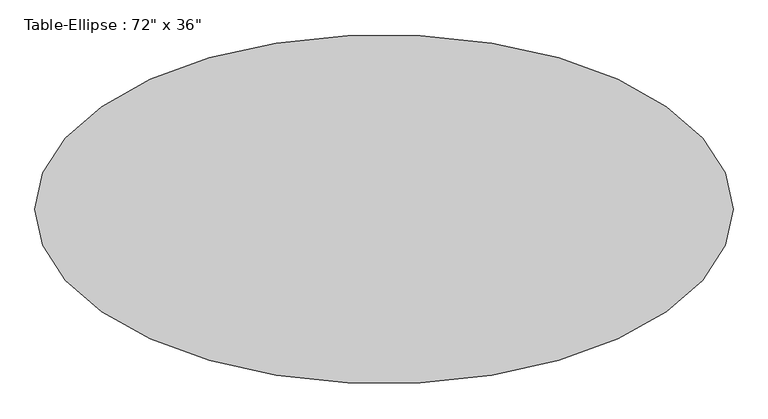
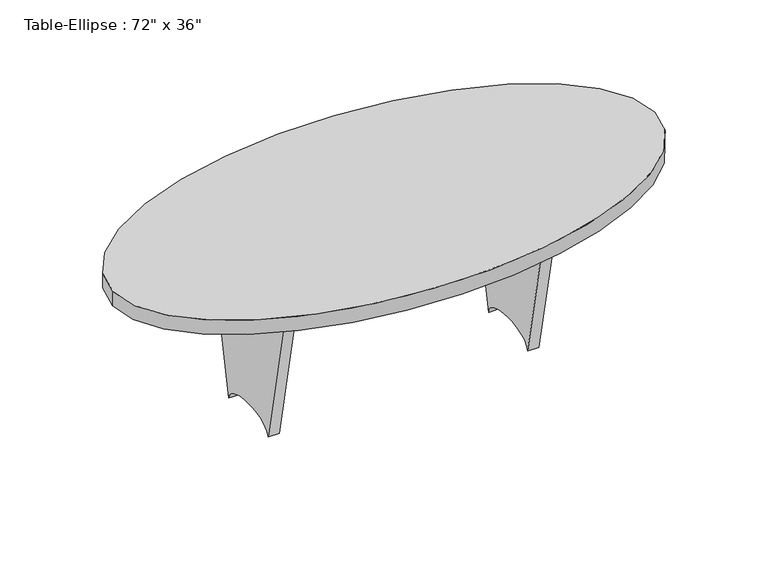
"""IFC4 building model written with IfcOpenShell, lengths in millimetres: furniture geometry."""

from ifc_helpers import new_model, si_unit, point, frame, origin, place, context, project, spatial, ellipse_curve, trimmed, source, transform, mapped, element, save
from ifc_brep_helpers import plane_surface, extruded_surface, advanced_brep


def furniture_c0716227(model_context):
    return source(origin(), model_context, "Body", "AdvancedBrep", [
        advanced_brep(
        [(-419.1, 19.05, 558.8), (419.1, 19.05, 558.8), (419.1, 19.05, 372.5333333), (-419.1, 19.05, 372.5333333), (-419.1, -19.05, 558.8), (-419.1, -19.05, 372.5333333), (419.1, -19.05, 372.5333333), (419.1, -19.05, 558.8)],
        [
            (0, 1),
            (1, 2),
            (2, 3, ellipse_curve(frame((0.0, 19.05, 372.5333333), z_axis=(0.0, -1.0, 0.0), x_axis=(1.0, 0.0, 0.0)), 419.1, 101.6)),
            (3, 0),
            (4, 5),
            (5, 6, ellipse_curve(frame((0.0, -19.05, 372.5333333), z_axis=(0.0, 1.0, 0.0), x_axis=(1.0, 0.0, 0.0)), 419.1, 101.6)),
            (6, 7),
            (7, 4),
            (0, 4),
            (7, 1),
            (6, 2),
            (5, 3),
        ],
        [
            plane_surface(frame((-419.1, 19.05, 558.8), z_axis=(0.0, 1.0, 0.0), x_axis=(1.0, 0.0, 0.0))),
            plane_surface(frame((-419.1, -19.05, 558.8), z_axis=(0.0, -1.0, 0.0), x_axis=(-1.0, 0.0, 0.0))),
            plane_surface(frame((-419.1, 19.05, 558.8), z_axis=(0.0, 0.0, 1.0), x_axis=(0.0, -1.0, 0.0))),
            plane_surface(frame((419.1, 19.05, 558.8), z_axis=(1.0, 0.0, 0.0), x_axis=(0.0, -1.0, 0.0))),
            extruded_surface(trimmed(ellipse_curve(frame((0.0, -57.15, 372.5333333), z_axis=(0.0, -1.0, 0.0), x_axis=(1.0, 0.0, 0.0)), 419.1, 101.6), [point((419.1, -57.15, 372.5333333))], [point((-419.1, -57.15, 372.5333333))], True, "CARTESIAN"), (0.0, 38.099999999999994, 0.0), 38.099999999999994),
            plane_surface(frame((-419.1, 19.05, 372.5333333), z_axis=(-1.0, 0.0, 0.0), x_axis=(0.0, -1.0, 0.0))),
        ],
        [
            (0, [[1, 2, 3, 4]]),
            (1, [[5, 6, 7, 8]]),
            (2, [[-1, 9, -8, 10]]),
            (3, [[-2, -10, -7, 11]]),
            (4, [[-3, -11, -6, 12]]),
            (5, [[-4, -12, -5, -9]]),
        ],
    ),
        advanced_brep(
        [(457.2, 228.6, 558.8), (457.2, -228.6, 558.8), (457.2, -114.3, 0.0), (457.2, 114.3, 0.0), (419.1, 228.6, 558.8), (419.1, 114.3, 0.0), (419.1, -114.3, 0.0), (419.1, -228.6, 558.8)],
        [
            (0, 1),
            (1, 2),
            (2, 3, ellipse_curve(frame((457.2, 0.0, 0.0), z_axis=(-1.0, 0.0, 0.0), x_axis=(0.0, 1.0, 0.0)), 114.3, 50.8)),
            (3, 0),
            (4, 5),
            (5, 6, ellipse_curve(frame((419.1, 0.0, 0.0), z_axis=(1.0, 0.0, 0.0), x_axis=(0.0, 1.0, 0.0)), 114.3, 50.8)),
            (6, 7),
            (7, 4),
            (0, 4),
            (7, 1),
            (6, 2),
            (5, 3),
        ],
        [
            plane_surface(frame((457.2, -228.6, 558.8), z_axis=(1.0, 0.0, 0.0), x_axis=(0.0, -1.0, 0.0))),
            plane_surface(frame((419.1, -228.6, 558.8), z_axis=(-1.0, 0.0, 0.0), x_axis=(0.0, 1.0, 0.0))),
            plane_surface(frame((457.2, 228.6, 558.8), z_axis=(0.0, 0.0, 1.0), x_axis=(-1.0, 0.0, 0.0))),
            plane_surface(frame((457.2, -228.6, 558.8), z_axis=(0.0, -0.9797149322825637, -0.20039623614871527), x_axis=(-1.0, 0.0, 0.0))),
            extruded_surface(trimmed(ellipse_curve(frame((381.0, 0.0, 0.0), z_axis=(-1.0, 0.0, 0.0), x_axis=(0.0, 1.0, 0.0)), 114.3, 50.8), [point((381.0, -114.3, 0.0))], [point((381.0, 114.3, 0.0))], True, "CARTESIAN"), (38.10000000000002, 0.0, 0.0), 38.10000000000002),
            plane_surface(frame((457.2, 114.3, 0.0), z_axis=(0.0, 0.9797149322825677, -0.2003962361486956), x_axis=(-1.0, 0.0, 0.0))),
        ],
        [
            (0, [[1, 2, 3, 4]]),
            (1, [[5, 6, 7, 8]]),
            (2, [[-1, 9, -8, 10]]),
            (3, [[-2, -10, -7, 11]]),
            (4, [[-3, -11, -6, 12]]),
            (5, [[-4, -12, -5, -9]]),
        ],
    ),
        advanced_brep(
        [(-419.1, 228.6, 558.8), (-419.1, -228.6, 558.8), (-419.1, -114.3, 0.0), (-419.1, 114.3, 0.0), (-457.2, 228.6, 558.8), (-457.2, 114.3, 0.0), (-457.2, -114.3, 0.0), (-457.2, -228.6, 558.8)],
        [
            (0, 1),
            (1, 2),
            (2, 3, ellipse_curve(frame((-419.1, 0.0, 0.0), z_axis=(-1.0, 0.0, 0.0), x_axis=(0.0, 1.0, 0.0)), 114.3, 50.8)),
            (3, 0),
            (4, 5),
            (5, 6, ellipse_curve(frame((-457.2, 0.0, 0.0), z_axis=(1.0, 0.0, 0.0), x_axis=(0.0, 1.0, 0.0)), 114.3, 50.8)),
            (6, 7),
            (7, 4),
            (0, 4),
            (7, 1),
            (6, 2),
            (5, 3),
        ],
        [
            plane_surface(frame((-419.1, -228.6, 558.8), z_axis=(1.0, 0.0, 0.0), x_axis=(0.0, -1.0, 0.0))),
            plane_surface(frame((-457.2, -228.6, 558.8), z_axis=(-1.0, 0.0, 0.0), x_axis=(0.0, 1.0, 0.0))),
            plane_surface(frame((-419.1, 228.6, 558.8), z_axis=(0.0, 0.0, 1.0), x_axis=(-1.0, 0.0, 0.0))),
            plane_surface(frame((-419.1, -228.6, 558.8), z_axis=(0.0, -0.979714932282564, -0.20039623614871366), x_axis=(-1.0, 0.0, 0.0))),
            extruded_surface(trimmed(ellipse_curve(frame((-495.3, 0.0, 0.0), z_axis=(-1.0, 0.0, 0.0), x_axis=(0.0, 1.0, 0.0)), 114.3, 50.8), [point((-495.3, -114.3, 0.0))], [point((-495.3, 114.3, 0.0))], True, "CARTESIAN"), (38.10000000000002, 0.0, 0.0), 38.10000000000002),
            plane_surface(frame((-419.1, 114.3, 0.0), z_axis=(0.0, 0.9797149322825663, -0.2003962361487023), x_axis=(-1.0, 0.0, 0.0))),
        ],
        [
            (0, [[1, 2, 3, 4]]),
            (1, [[5, 6, 7, 8]]),
            (2, [[-1, 9, -8, 10]]),
            (3, [[-2, -10, -7, 11]]),
            (4, [[-3, -11, -6, 12]]),
            (5, [[-4, -12, -5, -9]]),
        ],
    ),
        advanced_brep(
        [(-914.4, 0.0, 609.6), (914.4, 0.0, 609.6), (-914.4, 0.0, 558.8), (914.4, 0.0, 558.8)],
        [
            (0, 1, ellipse_curve(frame((0.0, 0.0, 609.6), z_axis=(0.0, 0.0, 1.0), x_axis=(1.0, 0.0, 0.0)), 914.4, 457.2)),
            (1, 0, ellipse_curve(frame((0.0, 0.0, 609.6), z_axis=(0.0, 0.0, 1.0), x_axis=(1.0, 0.0, 0.0)), 914.4, 457.2)),
            (2, 3, ellipse_curve(frame((0.0, 0.0, 558.8), z_axis=(0.0, 0.0, -1.0), x_axis=(1.0, 0.0, 0.0)), 914.4, 457.2)),
            (3, 2, ellipse_curve(frame((0.0, 0.0, 558.8), z_axis=(0.0, 0.0, -1.0), x_axis=(1.0, 0.0, 0.0)), 914.4, 457.2)),
            (0, 2),
            (3, 1),
        ],
        [
            plane_surface(frame((914.4, 0.0, 609.6), z_axis=(0.0, 0.0, 1.0), x_axis=(0.0, 1.0, 0.0))),
            plane_surface(frame((914.4, 0.0, 558.8), z_axis=(0.0, 0.0, -1.0), x_axis=(0.0, -1.0, 0.0))),
            extruded_surface(trimmed(ellipse_curve(frame((0.0, 0.0, 508.0), z_axis=(0.0, 0.0, 1.0), x_axis=(1.0, 0.0, 0.0)), 914.4, 457.2), [point((-914.4, 0.0, 508.0))], [point((914.4, 0.0, 508.0))], True, "CARTESIAN"), (0.0, 0.0, 50.799999999999955), 50.799999999999955),
            extruded_surface(trimmed(ellipse_curve(frame((0.0, 0.0, 508.0), z_axis=(0.0, 0.0, 1.0), x_axis=(1.0, 0.0, 0.0)), 914.4, 457.2), [point((914.4, 0.0, 508.0))], [point((-914.4, 0.0, 508.0))], True, "CARTESIAN"), (0.0, 0.0, 50.799999999999955), 50.799999999999955),
        ],
        [
            (0, [[1, 2]]),
            (1, [[3, 4]]),
            (2, [[-1, 5, -4, 6]]),
            (3, [[-2, -6, -3, -5]]),
        ],
    ),
    ])


if __name__ == "__main__":
    model = new_model("IFC4")
    model_context = context("Model", 3, world=origin())
    ifc_project = project(units=[si_unit("LENGTHUNIT", "METRE", prefix="MILLI")], contexts=[model_context])
    site = spatial("IfcSite", under=ifc_project)
    building = spatial("IfcBuilding", under=site)
    placement = place(None, origin())
    furniture_shape = furniture_c0716227(model_context)
    element("IfcFurniture", 1, ObjectType="Table-Ellipse : 72\" x 36\"", at=placement, inside=building, context=model_context, shape_type="MappedRepresentation", body=[
        mapped(furniture_shape, transform((0.0, 0.0, 0.0), x_axis=(1.0, 0.0, 0.0), y_axis=(0.0, 1.0, 0.0), z_axis=(0.0, 0.0, 1.0))),
    ])
    save(model, "model.ifc")

# Revit data of these elements
# Type "Table-Ellipse : 72\" x 36\""
#   Assembly Code = "E2020200"
#   Half Width = 1' - 6"
#   Half Length = 3' - 0"
#   Height = 2' - 0"
#   Length = 6' - 0"
#   Width = 3' - 0"
#   Base Material = Birch
#   Top Material = Wood - Teak
#   Default Elevation = 0
# Element 1 (IfcFurniture, "Table-Ellipse : 72\" x 36\"")
#   Materials on its faces: "Birch", "Wood - Teak"
# Materials
#   "Birch": class "Wood", colour RGB 224 178 126, transparency 0, Description = "Betula Alleghaniensis", Cost = 0
#   "Wood - Teak": class "Wood", colour RGB 145 112 90, transparency 0
